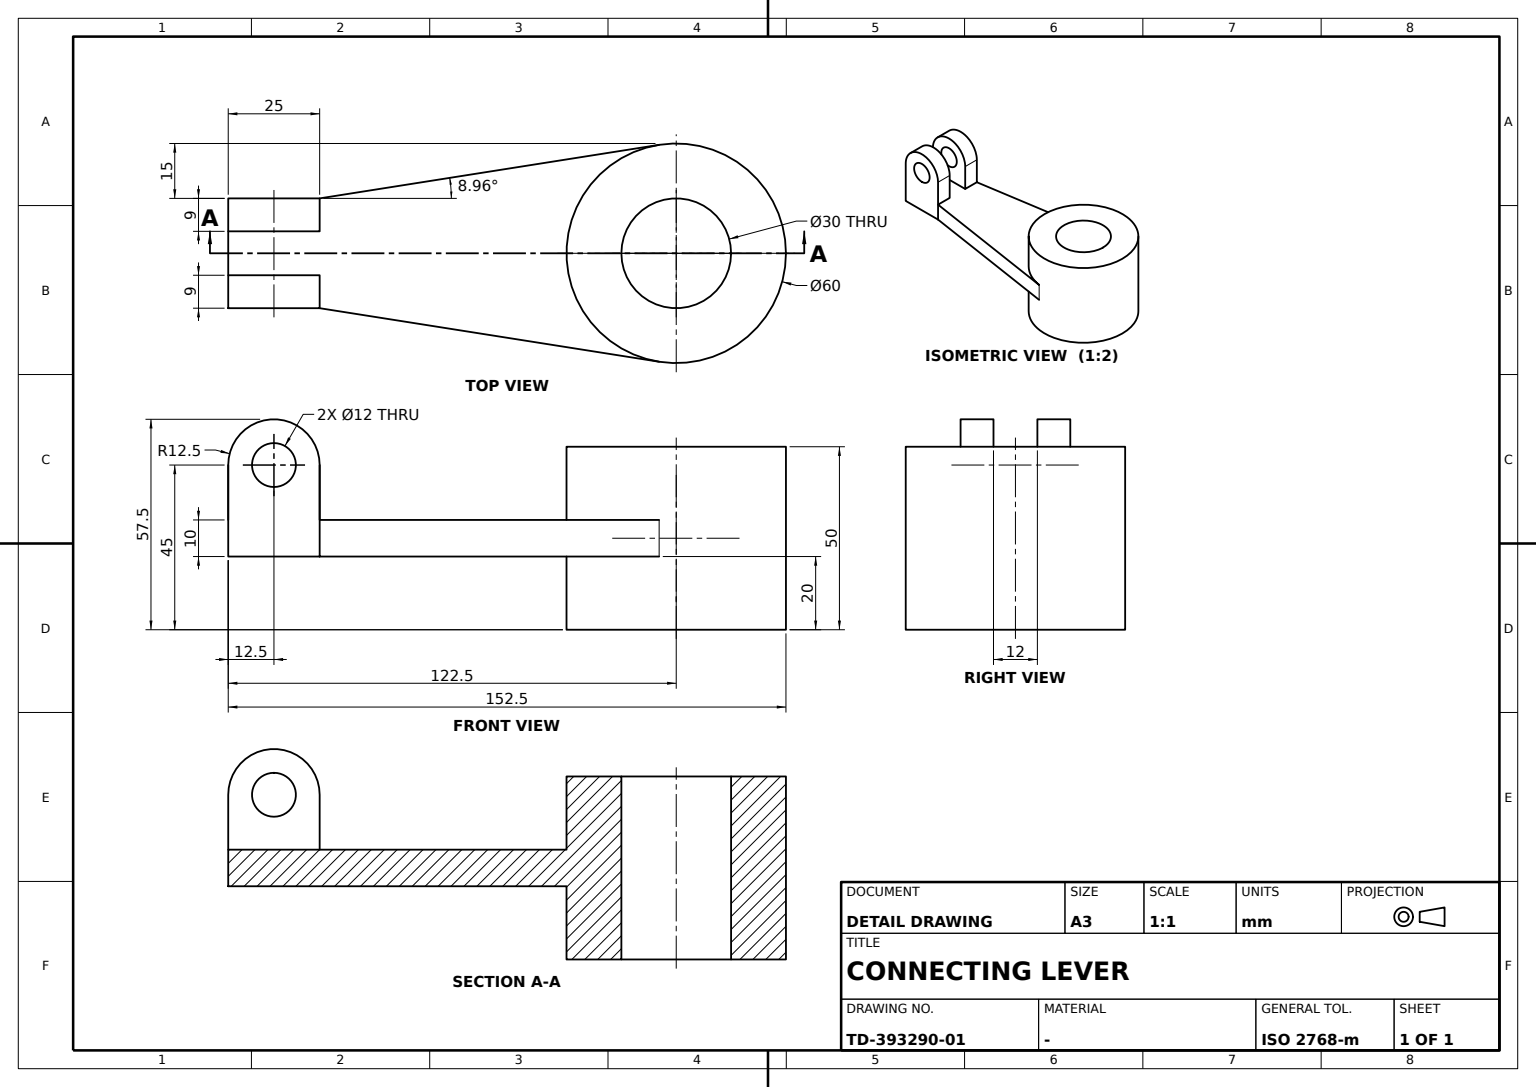
CATIA V5 part; units mm, degrees
sketch "Sketch1" plane through (0, 0, 0) normal (0, 0, 1) x (1, 0, 0)
  circle A0 centre (0, 0) radius 30
  circle A1 centre (0, 0) radius 15
  dimension "radius A1" = 15
  dimension "radius A0" = 30
extrude "Pad1" add sketch "Sketch1" along normal mid plane 50
sketch "Sketch3" plane through (0, 0, 0) normal (0, 0, 1) x (1, 0, 0)
  circle A0 centre (0, 0) radius 30 construction
  arc A1 (-4.6717, 29.634) -> (-4.6717, -29.634) centre (0, 0) ccw
  point P0 (-4.6717, 29.634)
  line L0 (-4.6717, 29.634) -> (-97.5, 15)
  point P1 (-97.5, 15)
  line L1 (-97.5, 15) -> (-122.5, 15)
  line L2 (-122.5, 15) -> (-122.5, -15)
  line L3 (-122.5, -15) -> (-97.5, -15)
  point P2 (-97.5, -15)
  point P3 (-4.6717, -29.634)
  line L4 (-4.6717, -29.634) -> (-97.5, -15)
  dimension "length L1" = 25
  dimension "distance L2 y axis" = 122.5
  dimension "length L3" = 25
  dimension "length L2" = 30
  constraint horizontal L1 x-axis
  constraint horizontal L3 x-axis
  constraint vertical L2 y-axis
  constraint symmetry L1 L3 x-axis
  constraint symmetry P1 P2 x-axis
  constraint symmetry P0 P3 x-axis
  constraint symmetry L0 L4 x-axis
  constraint tangency L0 A0
  constraint coincidence P0 A0
extrude "Pad2" add sketch "Sketch3" along normal mid plane 10
sketch "Sketch4" plane through (0, 15, 0) normal (0, 1, 0) x (-1, 0, 0)
  line L0 (97.5, 5) -> (122.5, 5)
  line L1 (122.5, 5) -> (122.5, 20)
  line L2 (97.5, 20) -> (97.5, 5)
  point P0 (122.5, 20)
  point P1 (97.5, 20)
  line L3 (122.5, -5) -> (122.5, 5) construction
  line L4 (97.5, 5) -> (122.5, 5) construction
  line L5 (97.5, -5) -> (97.5, 5) construction
  arc A0 (122.5, 20) -> (97.5, 20) centre (110, 20) ccw
  point P2 (110, 20)
  point P3 (122.5, 20)
  point P4 (97.5, 20)
  line L6 (97.5, -5) -> (122.5, -5) construction
  circle A1 centre (110, 20) radius 6
  dimension "distance P2 L6" = 25
  dimension "radius A1" = 6
  constraint horizontal L0 x-axis
  constraint vertical L1 y-axis
  constraint vertical L2 y-axis
  constraint coincidence L1 L3
  constraint coincidence L4 L0
  constraint coincidence L2 L5
  constraint coincidence P1 P4
  constraint coincidence P0 P3
  constraint tangency A0 L2
  constraint tangency A0 L1
  constraint concentricity A0 A1
extrude "Pad3" add sketch "Sketch4" against normal blind 9
mirror "Mirror1" about plane through (0, 0, 0) normal (0, 1, 0) of "Pad3"
sketch "Sketch2" plane through (0, 0, 0) normal (0, 0, 1) x (1, 0, 0)
